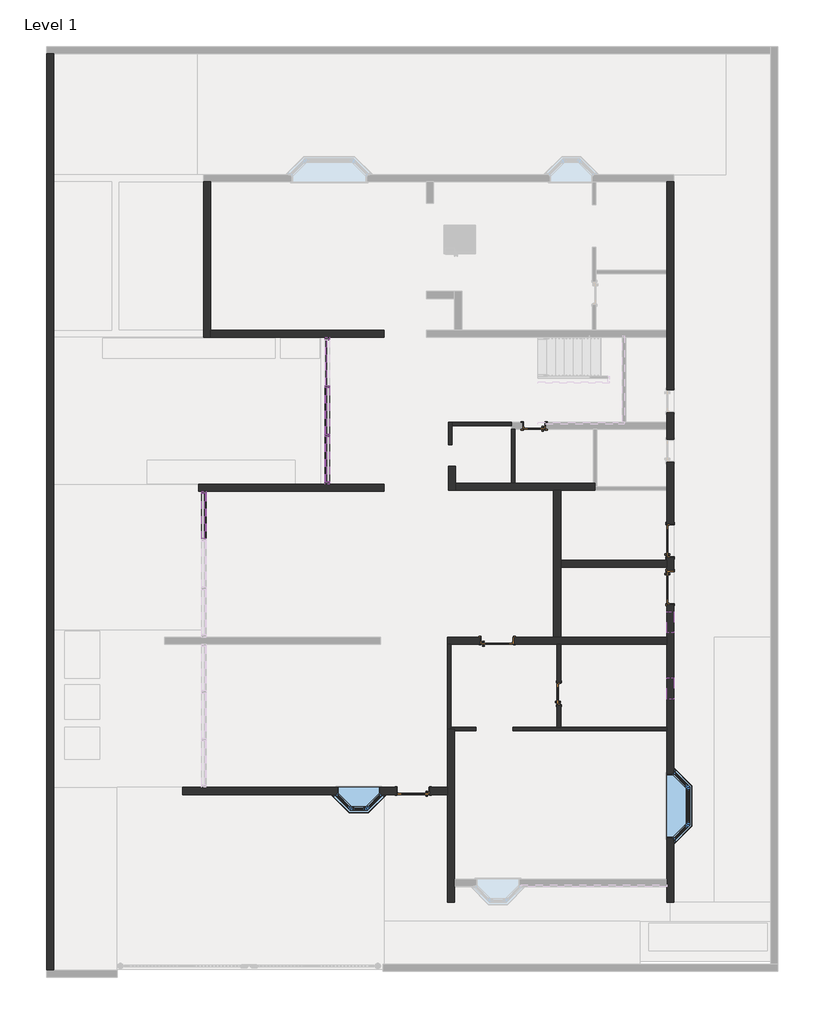
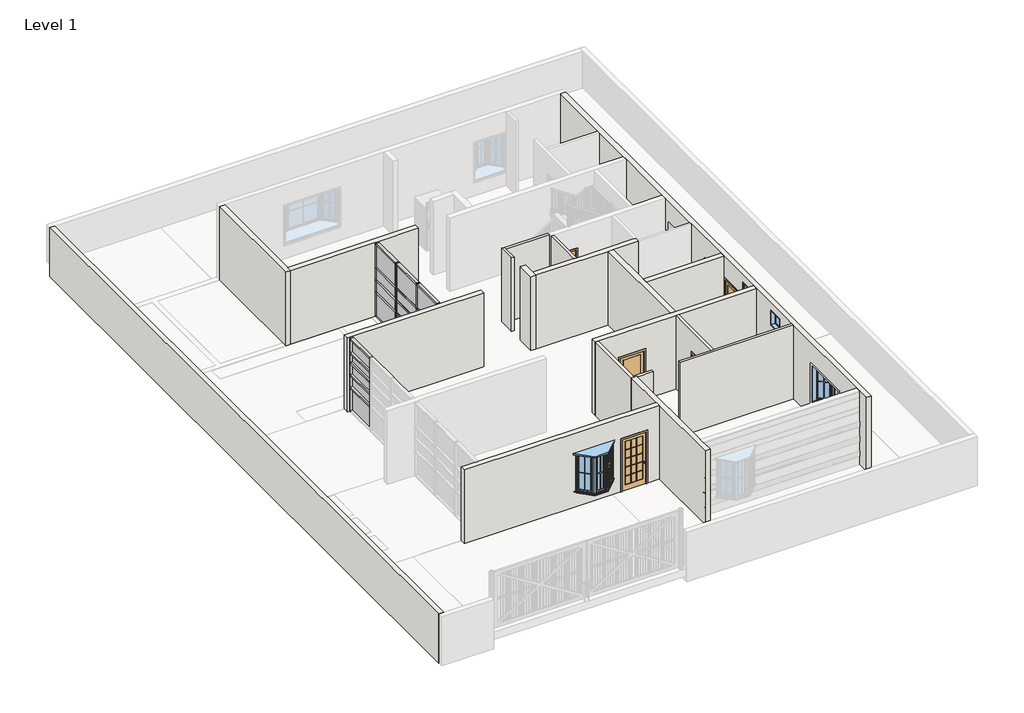
# One storey, part 3 of 5: 38 members, 19 walls, 17 plates, 6 doors, 4 windows.
"""IFC4 building model written with IfcOpenShell, lengths in millimetres."""

from ifc_helpers import new_model, si_unit, frame, origin, origin_with_axes, place, context, project, spatial, polyline, outline, extrude, faceted_brep, transform, mapped, element, save
from components import door_interior_single_1_panel_wood_5fe0af8f, door_interior_single_1_panel_wood_33af59b7, door_89b565b6, door_interior_single_1_panel_wood_secondary_door_3_x_7_9c4ddfbd, door_interior_single_1_panel_wood_secondary_door_3_x_7_1a936fe1, door_interior_single_full_glass_wood_main_glass_door_aaee7461, member_c0a82454, member_10605c90, member_f92b8aa2, member_90750a43, member_f9f7e124, member_161f4059, member_8e09d03a, member_7fd687a9, member_13061b82, member_37fe5cbd, member_7cfea1b5, member_47bfaf8a, system_panel_glazed_751bbe7c, system_panel_glazed_6c2f0e29, system_panel_glazed_201df7ca, system_panel_glazed_b8f86fea, system_panel_glazed_b72ced83, system_panel_glazed_b8338f5c, system_panel_glazed_2a12a50e, system_panel_glazed_2e6a26f2, window_6846e476, window_bay_casement_45_degree_angle_window_4_787d36ed, window_bay_casement_45_degree_angle_window_6_x4_737bffb6

model = new_model("IFC4")

# Units and contexts
model_context = context("Model", 3, world=origin())
ifc_project = project(units=[si_unit("LENGTHUNIT", "METRE", prefix="MILLI")], contexts=[model_context])

# Site, building, storey
site = spatial("IfcSite", under=ifc_project)
building = spatial("IfcBuilding", under=site)
storey = spatial("IfcBuildingStorey", under=building, Name="Level 1", Elevation=0.0)

# Doors
placement = place(None, origin())
door_interior_single_1_panel_wood_shape = door_interior_single_1_panel_wood_5fe0af8f(model_context)
element("IfcDoor", 1, ObjectType="Door-Interior-Single-1_Panel-Wood", at=placement, inside=storey, context=model_context, shape_type="MappedRepresentation", body=[
    mapped(door_interior_single_1_panel_wood_shape, transform((-41259.7380314, 3229.1336027, 0.0), x_axis=(-1.0, 0.0, 0.0), y_axis=(0.0, -1.0, 0.0), z_axis=(0.0, 0.0, 1.0))),
])
door_interior_single_1_panel_wood_2_shape = door_interior_single_1_panel_wood_33af59b7(model_context)
element("IfcDoor", 2, ObjectType="Door-Interior-Single-1_Panel-Wood", at=placement, inside=storey, context=model_context, shape_type="MappedRepresentation", body=[
    mapped(door_interior_single_1_panel_wood_2_shape, transform((-40551.7130314, -4463.8913973, 0.0), x_axis=(0.0, 1.0, 0.0), y_axis=(-1.0, 0.0, 0.0), z_axis=(0.0, 0.0, 1.0))),
])
door_shape = door_89b565b6(model_context)
element("IfcDoor", 3, ObjectType="Door-Interior-Single-1_Panel-Wood : 36\" x 80\"", at=placement, inside=storey, context=model_context, shape_type="MappedRepresentation", body=[
    mapped(door_shape, transform((-42326.5380314, -2943.0663973, 0.0), x_axis=(1.0, 0.0, 0.0), y_axis=(0.0, 1.0, 0.0), z_axis=(0.0, 0.0, 1.0))),
])
door_interior_single_1_panel_wood_secondary_door_3_x_7_shape = door_interior_single_1_panel_wood_secondary_door_3_x_7_9c4ddfbd(model_context)
element("IfcDoor", 4, ObjectType="Door-Interior-Single-1_Panel-Wood : SECONDARY DOOR 3' X 7'", at=placement, inside=storey, context=model_context, shape_type="MappedRepresentation", body=[
    mapped(door_interior_single_1_panel_wood_secondary_door_3_x_7_shape, transform((-37351.3130314, -69.6913973, 0.0), x_axis=(0.0, 1.0, 0.0), y_axis=(-1.0, 0.0, 0.0), z_axis=(0.0, 0.0, 1.0))),
])
door_interior_single_1_panel_wood_secondary_door_3_x_7_2_shape = door_interior_single_1_panel_wood_secondary_door_3_x_7_1a936fe1(model_context)
element("IfcDoor", 5, ObjectType="Door-Interior-Single-1_Panel-Wood : SECONDARY DOOR 3' X 7'", at=placement, inside=storey, context=model_context, shape_type="MappedRepresentation", body=[
    mapped(door_interior_single_1_panel_wood_secondary_door_3_x_7_2_shape, transform((-37351.3130314, -1415.8913973, 0.0), x_axis=(0.0, -1.0, 0.0), y_axis=(1.0, 0.0, 0.0), z_axis=(0.0, 0.0, 1.0))),
])
door_interior_single_full_glass_wood_main_glass_door_shape = door_interior_single_full_glass_wood_main_glass_door_aaee7461(model_context)
element("IfcDoor", 6, ObjectType="Door-Interior-Single-Full Glass-Wood : MAIN GLASS DOOR", at=placement, inside=storey, context=model_context, shape_type="MappedRepresentation", body=[
    mapped(door_interior_single_full_glass_wood_main_glass_door_shape, transform((-44739.5380314, -7261.0663973, 0.0), x_axis=(-1.0, 0.0, 0.0), y_axis=(0.0, -1.0, 0.0), z_axis=(0.0, 0.0, 1.0))),
])

# Members
member_shape = member_c0a82454(model_context)
element("IfcMember", 7, ObjectType="Rectangular Mullion : 2.5\" x 5\" rectangular", at=placement, inside=storey, context=model_context, shape_type="MappedRepresentation", body=[
    mapped(member_shape, transform((-47203.3380314, 5708.8086027, 3048.0), x_axis=(0.0, 0.0, 1.0), y_axis=(1.0, 0.0, 0.0), z_axis=(0.0, 1.0, 0.0))),
])
element("IfcMember", 8, ObjectType="Rectangular Mullion : 2.5\" x 5\" rectangular", at=placement, inside=storey, context=model_context, shape_type="MappedRepresentation", body=[
    mapped(member_shape, transform((-47203.3380314, 2929.6252695, 3048.0), x_axis=(0.0, 0.0, 1.0), y_axis=(1.0, 0.0, 0.0), z_axis=(0.0, 1.0, 0.0))),
])
element("IfcMember", 9, ObjectType="Rectangular Mullion : 2.5\" x 5\" rectangular", at=placement, inside=storey, context=model_context, shape_type="MappedRepresentation", body=[
    mapped(member_shape, transform((-47203.3380314, 1619.4086027, 0.0), x_axis=(0.0, 0.0, -1.0), y_axis=(1.0, 0.0, 0.0), z_axis=(0.0, -1.0, 0.0))),
])
element("IfcMember", 10, ObjectType="Rectangular Mullion : 2.5\" x 5\" rectangular", at=placement, inside=storey, context=model_context, shape_type="MappedRepresentation", body=[
    mapped(member_shape, transform((-47203.3380314, 4398.591936, 0.0), x_axis=(0.0, 0.0, -1.0), y_axis=(1.0, 0.0, 0.0), z_axis=(0.0, -1.0, 0.0))),
])
member_2_shape = member_10605c90(model_context)
element("IfcMember", 11, ObjectType="Rectangular Mullion : 2.5\" x 5\" rectangular", at=placement, inside=storey, context=model_context, shape_type="MappedRepresentation", body=[
    mapped(member_2_shape, transform((-47203.3380314, 4335.091936, 3048.0), x_axis=(0.0, 0.0, 1.0), y_axis=(1.0, 0.0, 0.0), z_axis=(0.0, 1.0, 0.0))),
])
element("IfcMember", 12, ObjectType="Rectangular Mullion : 2.5\" x 5\" rectangular", at=placement, inside=storey, context=model_context, shape_type="MappedRepresentation", body=[
    mapped(member_2_shape, transform((-47203.3380314, 2993.1252695, 0.0), x_axis=(0.0, 0.0, -1.0), y_axis=(1.0, 0.0, 0.0), z_axis=(0.0, -1.0, 0.0))),
])
member_3_shape = member_f92b8aa2(model_context)
element("IfcMember", 13, ObjectType="Rectangular Mullion : 2.5\" x 5\" rectangular", at=placement, inside=storey, context=model_context, shape_type="MappedRepresentation", body=[
    mapped(member_3_shape, transform((-47203.3380314, 4366.841936, 2032.0), x_axis=(0.0, 1.0, 0.0), y_axis=(1.0, 0.0, 0.0), z_axis=(0.0, 0.0, -1.0))),
])
element("IfcMember", 14, ObjectType="Rectangular Mullion : 2.5\" x 5\" rectangular", at=placement, inside=storey, context=model_context, shape_type="MappedRepresentation", body=[
    mapped(member_3_shape, transform((-47203.3380314, 2961.3752695, 2032.0), x_axis=(0.0, 1.0, 0.0), y_axis=(1.0, 0.0, 0.0), z_axis=(0.0, 0.0, -1.0))),
])
member_4_shape = member_90750a43(model_context)
element("IfcMember", 15, ObjectType="Rectangular Mullion : 2.5\" x 5\" rectangular", at=placement, inside=storey, context=model_context, shape_type="MappedRepresentation", body=[
    mapped(member_4_shape, transform((-47203.3380314, 4366.841936, 1016.0), x_axis=(0.0, 1.0, 0.0), y_axis=(1.0, 0.0, 0.0), z_axis=(0.0, 0.0, -1.0))),
])
element("IfcMember", 16, ObjectType="Rectangular Mullion : 2.5\" x 5\" rectangular", at=placement, inside=storey, context=model_context, shape_type="MappedRepresentation", body=[
    mapped(member_4_shape, transform((-47203.3380314, 4366.841936, 1524.0), x_axis=(0.0, 1.0, 0.0), y_axis=(1.0, 0.0, 0.0), z_axis=(0.0, 0.0, -1.0))),
])
element("IfcMember", 17, ObjectType="Rectangular Mullion : 2.5\" x 5\" rectangular", at=placement, inside=storey, context=model_context, shape_type="MappedRepresentation", body=[
    mapped(member_4_shape, transform((-47203.3380314, 2961.3752695, 1016.0), x_axis=(0.0, 1.0, 0.0), y_axis=(1.0, 0.0, 0.0), z_axis=(0.0, 0.0, -1.0))),
])
element("IfcMember", 18, ObjectType="Rectangular Mullion : 2.5\" x 5\" rectangular", at=placement, inside=storey, context=model_context, shape_type="MappedRepresentation", body=[
    mapped(member_4_shape, transform((-47203.3380314, 2961.3752695, 1524.0), x_axis=(0.0, 1.0, 0.0), y_axis=(1.0, 0.0, 0.0), z_axis=(0.0, 0.0, -1.0))),
])
element("IfcMember", 19, ObjectType="Rectangular Mullion : 2.5\" x 5\" rectangular", at=placement, inside=storey, context=model_context, shape_type="MappedRepresentation", body=[
    mapped(member_3_shape, transform((-47203.3380314, 4366.841936, 0.0), x_axis=(0.0, 1.0, 0.0), y_axis=(1.0, 0.0, 0.0), z_axis=(0.0, 0.0, -1.0))),
])
element("IfcMember", 20, ObjectType="Rectangular Mullion : 2.5\" x 5\" rectangular", at=placement, inside=storey, context=model_context, shape_type="MappedRepresentation", body=[
    mapped(member_3_shape, transform((-47203.3380314, 2961.3752695, 0.0), x_axis=(0.0, 1.0, 0.0), y_axis=(1.0, 0.0, 0.0), z_axis=(0.0, 0.0, -1.0))),
])
member_5_shape = member_f9f7e124(model_context)
element("IfcMember", 21, ObjectType="Rectangular Mullion : 2.5\" x 5\" rectangular", at=placement, inside=storey, context=model_context, shape_type="MappedRepresentation", body=[
    mapped(member_5_shape, transform((-47203.3380314, 2929.6252695, 1016.0), x_axis=(0.0, 0.0, 1.0), y_axis=(1.0, 0.0, 0.0), z_axis=(0.0, 1.0, 0.0))),
])
element("IfcMember", 22, ObjectType="Rectangular Mullion : 2.5\" x 5\" rectangular", at=placement, inside=storey, context=model_context, shape_type="MappedRepresentation", body=[
    mapped(member_5_shape, transform((-47203.3380314, 2929.6252695, 2032.0), x_axis=(0.0, 0.0, 1.0), y_axis=(1.0, 0.0, 0.0), z_axis=(0.0, 1.0, 0.0))),
])
element("IfcMember", 23, ObjectType="Rectangular Mullion : 2.5\" x 5\" rectangular", at=placement, inside=storey, context=model_context, shape_type="MappedRepresentation", body=[
    mapped(member_5_shape, transform((-47203.3380314, 2929.6252695, 1524.0), x_axis=(0.0, 0.0, 1.0), y_axis=(1.0, 0.0, 0.0), z_axis=(0.0, 1.0, 0.0))),
])
member_6_shape = member_161f4059(model_context)
element("IfcMember", 24, ObjectType="Rectangular Mullion : 2.5\" x 5\" rectangular", at=placement, inside=storey, context=model_context, shape_type="MappedRepresentation", body=[
    mapped(member_6_shape, transform((-47203.3380314, 4335.091936, 1016.0), x_axis=(0.0, 0.0, 1.0), y_axis=(1.0, 0.0, 0.0), z_axis=(0.0, 1.0, 0.0))),
])
element("IfcMember", 25, ObjectType="Rectangular Mullion : 2.5\" x 5\" rectangular", at=placement, inside=storey, context=model_context, shape_type="MappedRepresentation", body=[
    mapped(member_6_shape, transform((-47203.3380314, 4335.091936, 2032.0), x_axis=(0.0, 0.0, 1.0), y_axis=(1.0, 0.0, 0.0), z_axis=(0.0, 1.0, 0.0))),
])
element("IfcMember", 26, ObjectType="Rectangular Mullion : 2.5\" x 5\" rectangular", at=placement, inside=storey, context=model_context, shape_type="MappedRepresentation", body=[
    mapped(member_6_shape, transform((-47203.3380314, 4335.091936, 1524.0), x_axis=(0.0, 0.0, 1.0), y_axis=(1.0, 0.0, 0.0), z_axis=(0.0, 1.0, 0.0))),
])
member_7_shape = member_8e09d03a(model_context)
element("IfcMember", 27, ObjectType="Rectangular Mullion : 2.5\" x 5\" rectangular", at=placement, inside=storey, context=model_context, shape_type="MappedRepresentation", body=[
    mapped(member_7_shape, transform((-47203.3380314, 5772.3086027, 0.0), x_axis=(0.0, 1.0, 0.0), y_axis=(1.0, 0.0, 0.0), z_axis=(0.0, 0.0, -1.0))),
])
element("IfcMember", 28, ObjectType="Rectangular Mullion : 2.5\" x 5\" rectangular", at=placement, inside=storey, context=model_context, shape_type="MappedRepresentation", body=[
    mapped(member_7_shape, transform((-47203.3380314, 1555.9086027, 3048.0), x_axis=(0.0, -1.0, 0.0), y_axis=(1.0, 0.0, 0.0), z_axis=(0.0, 0.0, 1.0))),
])
member_8_shape = member_7fd687a9(model_context)
element("IfcMember", 29, ObjectType="Rectangular Mullion : 2.5\" x 5\" rectangular", at=placement, inside=storey, context=model_context, shape_type="MappedRepresentation", body=[
    mapped(member_8_shape, transform((-47203.3380314, 5772.3086027, 1016.0), x_axis=(0.0, 1.0, 0.0), y_axis=(1.0, 0.0, 0.0), z_axis=(0.0, 0.0, -1.0))),
])
element("IfcMember", 30, ObjectType="Rectangular Mullion : 2.5\" x 5\" rectangular", at=placement, inside=storey, context=model_context, shape_type="MappedRepresentation", body=[
    mapped(member_8_shape, transform((-47203.3380314, 5772.3086027, 1524.0), x_axis=(0.0, 1.0, 0.0), y_axis=(1.0, 0.0, 0.0), z_axis=(0.0, 0.0, -1.0))),
])
element("IfcMember", 31, ObjectType="Rectangular Mullion : 2.5\" x 5\" rectangular", at=placement, inside=storey, context=model_context, shape_type="MappedRepresentation", body=[
    mapped(member_7_shape, transform((-47203.3380314, 1555.9086027, 1016.0), x_axis=(0.0, -1.0, 0.0), y_axis=(1.0, 0.0, 0.0), z_axis=(0.0, 0.0, 1.0))),
])
element("IfcMember", 32, ObjectType="Rectangular Mullion : 2.5\" x 5\" rectangular", at=placement, inside=storey, context=model_context, shape_type="MappedRepresentation", body=[
    mapped(member_8_shape, transform((-47203.3380314, 1555.9086027, 2032.0), x_axis=(0.0, -1.0, 0.0), y_axis=(1.0, 0.0, 0.0), z_axis=(0.0, 0.0, 1.0))),
])
element("IfcMember", 33, ObjectType="Rectangular Mullion : 2.5\" x 5\" rectangular", at=placement, inside=storey, context=model_context, shape_type="MappedRepresentation", body=[
    mapped(member_8_shape, transform((-47203.3380314, 1555.9086027, 1524.0), x_axis=(0.0, -1.0, 0.0), y_axis=(1.0, 0.0, 0.0), z_axis=(0.0, 0.0, 1.0))),
])
element("IfcMember", 34, ObjectType="Rectangular Mullion : 2.5\" x 5\" rectangular", at=placement, inside=storey, context=model_context, shape_type="MappedRepresentation", body=[
    mapped(member_7_shape, transform((-47203.3380314, 5772.3086027, 2032.0), x_axis=(0.0, 1.0, 0.0), y_axis=(1.0, 0.0, 0.0), z_axis=(0.0, 0.0, -1.0))),
])
member_9_shape = member_13061b82(model_context)
element("IfcMember", 35, ObjectType="Rectangular Mullion : 2.5\" x 5\" rectangular", at=placement, inside=storey, context=model_context, shape_type="MappedRepresentation", body=[
    mapped(member_9_shape, transform((-50759.3380314, 1289.2086027, 3048.0), x_axis=(0.0, 0.0, 1.0), y_axis=(1.0, 0.0, 0.0), z_axis=(0.0, 1.0, 0.0))),
])
member_10_shape = member_37fe5cbd(model_context)
element("IfcMember", 36, ObjectType="Rectangular Mullion : 2.5\" x 5\" rectangular", at=placement, inside=storey, context=model_context, shape_type="MappedRepresentation", body=[
    mapped(member_10_shape, transform((-50759.3380314, 1289.2086027, 1016.0), x_axis=(0.0, 0.0, 1.0), y_axis=(1.0, 0.0, 0.0), z_axis=(0.0, 1.0, 0.0))),
])
element("IfcMember", 37, ObjectType="Rectangular Mullion : 2.5\" x 5\" rectangular", at=placement, inside=storey, context=model_context, shape_type="MappedRepresentation", body=[
    mapped(member_10_shape, transform((-50759.3380314, 1289.2086027, 2032.0), x_axis=(0.0, 0.0, 1.0), y_axis=(1.0, 0.0, 0.0), z_axis=(0.0, 1.0, 0.0))),
])
element("IfcMember", 38, ObjectType="Rectangular Mullion : 2.5\" x 5\" rectangular", at=placement, inside=storey, context=model_context, shape_type="MappedRepresentation", body=[
    mapped(member_10_shape, transform((-50759.3380314, 1289.2086027, 1524.0), x_axis=(0.0, 0.0, 1.0), y_axis=(1.0, 0.0, 0.0), z_axis=(0.0, 1.0, 0.0))),
])
element("IfcMember", 39, ObjectType="Rectangular Mullion : 2.5\" x 5\" rectangular", at=placement, inside=storey, context=model_context, shape_type="MappedRepresentation", body=[
    mapped(member_10_shape, transform((-50759.3380314, 1289.2086027, 2438.4), x_axis=(0.0, 0.0, 1.0), y_axis=(1.0, 0.0, 0.0), z_axis=(0.0, 1.0, 0.0))),
])
element("IfcMember", 40, ObjectType="Rectangular Mullion : 2.5\" x 5\" rectangular", at=placement, inside=storey, context=model_context, shape_type="MappedRepresentation", body=[
    mapped(member_7_shape, transform((-50759.3380314, 1352.7086027, 0.0), x_axis=(0.0, 1.0, 0.0), y_axis=(1.0, 0.0, 0.0), z_axis=(0.0, 0.0, -1.0))),
])
element("IfcMember", 41, ObjectType="Rectangular Mullion : 2.5\" x 5\" rectangular", at=placement, inside=storey, context=model_context, shape_type="MappedRepresentation", body=[
    mapped(member_8_shape, transform((-50759.3380314, 1352.7086027, 1016.0), x_axis=(0.0, 1.0, 0.0), y_axis=(1.0, 0.0, 0.0), z_axis=(0.0, 0.0, -1.0))),
])
element("IfcMember", 42, ObjectType="Rectangular Mullion : 2.5\" x 5\" rectangular", at=placement, inside=storey, context=model_context, shape_type="MappedRepresentation", body=[
    mapped(member_8_shape, transform((-50759.3380314, 1352.7086027, 1524.0), x_axis=(0.0, 1.0, 0.0), y_axis=(1.0, 0.0, 0.0), z_axis=(0.0, 0.0, -1.0))),
])
member_11_shape = member_7cfea1b5(model_context)
element("IfcMember", 43, ObjectType="Rectangular Mullion : 2.5\" x 5\" rectangular", at=placement, inside=storey, context=model_context, shape_type="MappedRepresentation", body=[
    mapped(member_11_shape, transform((-50759.3380314, 1352.7086027, 2032.0), x_axis=(0.0, 1.0, 0.0), y_axis=(1.0, 0.0, 0.0), z_axis=(0.0, 0.0, -1.0))),
])
member_12_shape = member_47bfaf8a(model_context)
element("IfcMember", 44, ObjectType="Rectangular Mullion : 2.5\" x 5\" rectangular", at=placement, inside=storey, context=model_context, shape_type="MappedRepresentation", body=[
    mapped(member_12_shape, transform((-50759.3380314, 1352.7086027, 2438.4), x_axis=(0.0, 1.0, 0.0), y_axis=(1.0, 0.0, 0.0), z_axis=(0.0, 0.0, -1.0))),
])

# Plates
system_panel_glazed_shape = system_panel_glazed_751bbe7c(model_context)
element("IfcPlate", 45, ObjectType="System Panel : Glazed", at=placement, inside=storey, context=model_context, shape_type="MappedRepresentation", body=[
    mapped(system_panel_glazed_shape, transform((-47203.3380314, 2274.5169361, 63.5), x_axis=(0.0, 1.0, 0.0), y_axis=(-1.0, 0.0, 0.0), z_axis=(0.0, 0.0, 1.0))),
])
element("IfcPlate", 46, ObjectType="System Panel : Glazed", at=placement, inside=storey, context=model_context, shape_type="MappedRepresentation", body=[
    mapped(system_panel_glazed_shape, transform((-47203.3380314, 5053.7002694, 63.5), x_axis=(0.0, 1.0, 0.0), y_axis=(-1.0, 0.0, 0.0), z_axis=(0.0, 0.0, 1.0))),
])
element("IfcPlate", 47, ObjectType="System Panel : Glazed", at=placement, inside=storey, context=model_context, shape_type="MappedRepresentation", body=[
    mapped(system_panel_glazed_shape, transform((-47203.3380314, 2274.5169361, 2063.75), x_axis=(0.0, 1.0, 0.0), y_axis=(-1.0, 0.0, 0.0), z_axis=(0.0, 0.0, 1.0))),
])
element("IfcPlate", 48, ObjectType="System Panel : Glazed", at=placement, inside=storey, context=model_context, shape_type="MappedRepresentation", body=[
    mapped(system_panel_glazed_shape, transform((-47203.3380314, 5053.7002694, 2063.75), x_axis=(0.0, 1.0, 0.0), y_axis=(-1.0, 0.0, 0.0), z_axis=(0.0, 0.0, 1.0))),
])
system_panel_glazed_2_shape = system_panel_glazed_6c2f0e29(model_context)
element("IfcPlate", 49, ObjectType="System Panel : Glazed", at=placement, inside=storey, context=model_context, shape_type="MappedRepresentation", body=[
    mapped(system_panel_glazed_2_shape, transform((-47203.3380314, 3664.1086027, 63.5), x_axis=(0.0, 1.0, 0.0), y_axis=(-1.0, 0.0, 0.0), z_axis=(0.0, 0.0, 1.0))),
])
element("IfcPlate", 50, ObjectType="System Panel : Glazed", at=placement, inside=storey, context=model_context, shape_type="MappedRepresentation", body=[
    mapped(system_panel_glazed_2_shape, transform((-47203.3380314, 3664.1086027, 2063.75), x_axis=(0.0, 1.0, 0.0), y_axis=(-1.0, 0.0, 0.0), z_axis=(0.0, 0.0, 1.0))),
])
system_panel_glazed_3_shape = system_panel_glazed_201df7ca(model_context)
element("IfcPlate", 51, ObjectType="System Panel : Glazed", at=placement, inside=storey, context=model_context, shape_type="MappedRepresentation", body=[
    mapped(system_panel_glazed_3_shape, transform((-47203.3380314, 2274.5169361, 1047.75), x_axis=(0.0, 1.0, 0.0), y_axis=(-1.0, 0.0, 0.0), z_axis=(0.0, 0.0, 1.0))),
])
element("IfcPlate", 52, ObjectType="System Panel : Glazed", at=placement, inside=storey, context=model_context, shape_type="MappedRepresentation", body=[
    mapped(system_panel_glazed_3_shape, transform((-47203.3380314, 5053.7002694, 1047.75), x_axis=(0.0, 1.0, 0.0), y_axis=(-1.0, 0.0, 0.0), z_axis=(0.0, 0.0, 1.0))),
])
element("IfcPlate", 53, ObjectType="System Panel : Glazed", at=placement, inside=storey, context=model_context, shape_type="MappedRepresentation", body=[
    mapped(system_panel_glazed_3_shape, transform((-47203.3380314, 2274.5169361, 1555.75), x_axis=(0.0, 1.0, 0.0), y_axis=(-1.0, 0.0, 0.0), z_axis=(0.0, 0.0, 1.0))),
])
element("IfcPlate", 54, ObjectType="System Panel : Glazed", at=placement, inside=storey, context=model_context, shape_type="MappedRepresentation", body=[
    mapped(system_panel_glazed_3_shape, transform((-47203.3380314, 5053.7002694, 1555.75), x_axis=(0.0, 1.0, 0.0), y_axis=(-1.0, 0.0, 0.0), z_axis=(0.0, 0.0, 1.0))),
])
system_panel_glazed_4_shape = system_panel_glazed_b8f86fea(model_context)
element("IfcPlate", 55, ObjectType="System Panel : Glazed", at=placement, inside=storey, context=model_context, shape_type="MappedRepresentation", body=[
    mapped(system_panel_glazed_4_shape, transform((-47203.3380314, 3664.1086027, 1047.75), x_axis=(0.0, 1.0, 0.0), y_axis=(-1.0, 0.0, 0.0), z_axis=(0.0, 0.0, 1.0))),
])
element("IfcPlate", 56, ObjectType="System Panel : Glazed", at=placement, inside=storey, context=model_context, shape_type="MappedRepresentation", body=[
    mapped(system_panel_glazed_4_shape, transform((-47203.3380314, 3664.1086027, 1555.75), x_axis=(0.0, 1.0, 0.0), y_axis=(-1.0, 0.0, 0.0), z_axis=(0.0, 0.0, 1.0))),
])
system_panel_glazed_5_shape = system_panel_glazed_b72ced83(model_context)
element("IfcPlate", 57, ObjectType="System Panel : Glazed", at=placement, inside=storey, context=model_context, shape_type="MappedRepresentation", body=[
    mapped(system_panel_glazed_5_shape, transform((-50759.3380314, 638.3336027, 63.5), x_axis=(0.0, 1.0, 0.0), y_axis=(-1.0, 0.0, 0.0), z_axis=(0.0, 0.0, 1.0))),
])
system_panel_glazed_6_shape = system_panel_glazed_b8338f5c(model_context)
element("IfcPlate", 58, ObjectType="System Panel : Glazed", at=placement, inside=storey, context=model_context, shape_type="MappedRepresentation", body=[
    mapped(system_panel_glazed_6_shape, transform((-50759.3380314, 638.3336027, 1047.75), x_axis=(0.0, 1.0, 0.0), y_axis=(-1.0, 0.0, 0.0), z_axis=(0.0, 0.0, 1.0))),
])
element("IfcPlate", 59, ObjectType="System Panel : Glazed", at=placement, inside=storey, context=model_context, shape_type="MappedRepresentation", body=[
    mapped(system_panel_glazed_6_shape, transform((-50759.3380314, 638.3336027, 1555.75), x_axis=(0.0, 1.0, 0.0), y_axis=(-1.0, 0.0, 0.0), z_axis=(0.0, 0.0, 1.0))),
])
system_panel_glazed_7_shape = system_panel_glazed_2a12a50e(model_context)
element("IfcPlate", 60, ObjectType="System Panel : Glazed", at=placement, inside=storey, context=model_context, shape_type="MappedRepresentation", body=[
    mapped(system_panel_glazed_7_shape, transform((-50759.3380314, 638.3336027, 2063.75), x_axis=(0.0, 1.0, 0.0), y_axis=(-1.0, 0.0, 0.0), z_axis=(0.0, 0.0, 1.0))),
])
system_panel_glazed_8_shape = system_panel_glazed_2e6a26f2(model_context)
element("IfcPlate", 61, ObjectType="System Panel : Glazed", at=placement, inside=storey, context=model_context, shape_type="MappedRepresentation", body=[
    mapped(system_panel_glazed_8_shape, transform((-50759.3380314, 638.3336027, 2470.15), x_axis=(0.0, 1.0, 0.0), y_axis=(-1.0, 0.0, 0.0), z_axis=(0.0, 0.0, 1.0))),
])

# Walls
element("IfcWall", 62, ObjectType="INNER WALL 4\"", at=placement, inside=storey, context=model_context, shape_type="SweptSolid", body=[
    extrude(outline(polyline([(-41920.1380314, 1581.3086027), (-41920.1380314, 3130.7086027), (-41818.5380314, 3130.7086027), (-41818.5380314, 1581.3086027), (-41920.1380314, 1581.3086027)])), origin_with_axes(), (0.0, 0.0, 1.0), 3048.0),
])
element("IfcWall", 63, ObjectType="INNER WALL 4\"", at=placement, inside=storey, context=model_context, shape_type="Brep", body=[
    faceted_brep([(-43748.9380314, -3041.4913973, 0.0), (-43748.9380314, -5479.8913973, 0.0), (-43748.9380314, -5479.8913973, 3048.0), (-43748.9380314, -3041.4913973, 3048.0), (-43647.3380314, -3041.4913973, 0.0), (-43647.3380314, -3041.4913973, 3048.0), (-43647.3380314, -5429.0913973, 3048.0), (-43647.3380314, -5479.8913973, 3048.0), (-43647.3380314, -5479.8913973, 0.0), (-43647.3380314, -5429.0913973, 0.0)], [[[0, 1, 2, 3]], [[4, 5, 6, 7, 8, 9]], [[1, 0, 4, 9, 8]], [[2, 1, 8, 7]], [[3, 2, 7, 6, 5]], [[0, 3, 5, 4]]]),
])
element("IfcWall", 64, ObjectType="INNER WALL 4\"", at=placement, inside=storey, context=model_context, shape_type="SweptSolid", body=[
    extrude(outline(polyline([(-43647.3380314, -5429.0913973), (-42936.1380314, -5429.0913973), (-42936.1380314, -5530.6913973), (-43545.7380314, -5530.6913973), (-43545.7380314, -5479.8913973), (-43647.3380314, -5479.8913973), (-43647.3380314, -5429.0913973)])), origin_with_axes(), (0.0, 0.0, 1.0), 3048.0),
])
element("IfcWall", 65, ObjectType="INNER WALL 4\"", at=placement, inside=storey, context=model_context, shape_type="Brep", body=[
    faceted_brep([(-41869.3380314, -5530.6913973, 0.0), (-37449.7380314, -5530.6913973, 0.0), (-37449.7380314, -5530.6913973, 3048.0), (-41869.3380314, -5530.6913973, 3048.0), (-41869.3380314, -5429.0913973, 0.0), (-41869.3380314, -5429.0913973, 3048.0), (-40599.3380314, -5429.0913973, 3048.0), (-40497.7380314, -5429.0913973, 3048.0), (-37449.7380314, -5429.0913973, 3048.0), (-37449.7380314, -5429.0913973, 0.0), (-40497.7380314, -5429.0913973, 0.0), (-40599.3380314, -5429.0913973, 0.0)], [[[0, 1, 2, 3]], [[4, 5, 6, 7, 8, 9, 10, 11]], [[1, 0, 4, 11, 10, 9]], [[3, 2, 8, 7, 6, 5]], [[0, 3, 5, 4]], [[2, 1, 9, 8]]]),
])
element("IfcWall", 66, ObjectType="INNER WALL 4\"", at=placement, inside=storey, context=model_context, shape_type="SweptSolid", body=[
    extrude(outline(polyline([(-5429.0913973, 3048.0), (-3041.4913973, 3048.0), (-3041.4913973, 0.0), (-4133.6913973, 0.0), (-4133.6913973, 2159.0), (-4794.0913973, 2159.0), (-4794.0913973, 0.0), (-5429.0913973, 0.0), (-5429.0913973, 3048.0)])), frame((-40599.3380314, 0.0, 0.0), z_axis=(1.0, 0.0, 0.0), x_axis=(0.0, 1.0, 0.0)), (0.0, 0.0, 1.0), 101.6),
])
element("IfcWall", 67, ObjectType="INNER WALL 4\"", at=placement, inside=storey, context=model_context, shape_type="Brep", body=[
    faceted_brep([(-43621.9380314, 2686.2086027, 0.0), (-43621.9380314, 3232.3086027, 0.0), (-43621.9380314, 3333.9086027, 0.0), (-43621.9380314, 3333.9086027, 3048.0), (-43621.9380314, 3232.3086027, 3048.0), (-43621.9380314, 2686.2086027, 3048.0), (-43723.5380314, 2686.2086027, 0.0), (-43723.5380314, 2686.2086027, 3048.0), (-43723.5380314, 3333.9086027, 3048.0), (-43723.5380314, 3333.9086027, 0.0)], [[[0, 1, 2, 3, 4, 5]], [[6, 7, 8, 9]], [[2, 1, 0, 6, 9]], [[5, 4, 3, 8, 7]], [[0, 5, 7, 6]], [[3, 2, 9, 8]]]),
])
element("IfcWall", 68, ObjectType="INNER WALL 4\"", at=placement, inside=storey, context=model_context, shape_type="SweptSolid", body=[
    extrude(outline(polyline([(-41920.1380314, 3232.3086027), (-43621.9380314, 3232.3086027), (-43621.9380314, 3333.9086027), (-41920.1380314, 3333.9086027), (-41920.1380314, 3232.3086027)])), origin_with_axes(), (0.0, 0.0, 1.0), 3048.0),
])
element("IfcWall", 69, ObjectType="OUTER WALL 8\"", at=placement, inside=storey, context=model_context, shape_type="Brep", body=[
    faceted_brep([(-50759.3380314, 10242.7086027, 0.0), (-50759.3380314, 5772.3086027, 0.0), (-50759.3380314, 5772.3086027, 3048.0), (-50759.3380314, 10242.7086027, 3048.0), (-50556.1380314, 10242.7086027, 0.0), (-50556.1380314, 10242.7086027, 3048.0), (-50556.1380314, 5975.5086027, 3048.0), (-50556.1380314, 5772.3086027, 3048.0), (-50556.1380314, 5772.3086027, 0.0), (-50556.1380314, 5975.5086027, 0.0)], [[[0, 1, 2, 3]], [[4, 5, 6, 7, 8, 9]], [[1, 0, 4, 9, 8]], [[3, 2, 7, 6, 5]], [[0, 3, 5, 4]], [[2, 1, 8, 7]]]),
])
element("IfcWall", 70, ObjectType="OUTER WALL 8\"", at=placement, inside=storey, context=model_context, shape_type="Brep", body=[
    faceted_brep([(-45577.7380314, 5975.5086027, 0.0), (-50556.1380314, 5975.5086027, 0.0), (-50556.1380314, 5975.5086027, 3048.0), (-45577.7380314, 5975.5086027, 3048.0), (-45577.7380314, 5772.3086027, 0.0), (-45577.7380314, 5772.3086027, 3048.0), (-47203.3380314, 5772.3086027, 3048.0), (-47406.5380314, 5772.3086027, 3048.0), (-50556.1380314, 5772.3086027, 3048.0), (-50556.1380314, 5772.3086027, 0.0), (-47406.5380314, 5772.3086027, 0.0), (-47203.3380314, 5772.3086027, 0.0)], [[[0, 1, 2, 3]], [[4, 5, 6, 7, 8, 9, 10, 11]], [[1, 0, 4, 11, 10, 9]], [[3, 2, 8, 7, 6, 5]], [[0, 3, 5, 4]], [[2, 1, 9, 8]]]),
])
element("IfcWall", 71, ObjectType="OUTER WALL 8\"", at=placement, inside=storey, context=model_context, shape_type="SweptSolid", body=[
    extrude(outline(polyline([(-50905.3880314, 1555.9086027), (-45577.7380314, 1555.9086027), (-45577.7380314, 1352.7086027), (-50905.3880314, 1352.7086027), (-50905.3880314, 1555.9086027)])), origin_with_axes(), (0.0, 0.0, 1.0), 3048.0),
])
element("IfcWall", 72, ObjectType="OUTER WALL 8\"", at=placement, inside=storey, context=model_context, shape_type="Brep", body=[
    faceted_brep([(-43748.9380314, -7359.4913973, 3048.0), (-51368.9380314, -7359.4913973, 3048.0), (-51368.9380314, -7359.4913973, 0.0), (-45222.1380314, -7359.4913973, 0.0), (-45222.1380314, -7359.4913973, 2159.0), (-44256.9380314, -7359.4913973, 2159.0), (-44256.9380314, -7359.4913973, 0.0), (-43748.9380314, -7359.4913973, 0.0), (-46960.6294401, -7359.4913973, 2184.4), (-45642.6466227, -7359.4913973, 2184.4), (-45642.6466227, -7359.4913973, 609.6), (-46960.6294401, -7359.4913973, 609.6), (-51368.9380314, -7156.2913973, 3048.0), (-43748.9380314, -7156.2913973, 3048.0), (-43748.9380314, -7156.2913973, 0.0), (-44256.9380314, -7156.2913973, 0.0), (-44256.9380314, -7156.2913973, 2159.0), (-45222.1380314, -7156.2913973, 2159.0), (-45222.1380314, -7156.2913973, 0.0), (-51368.9380314, -7156.2913973, 0.0), (-45692.0380314, -7156.2913973, 2184.4), (-46911.2380314, -7156.2913973, 2184.4), (-46911.2380314, -7156.2913973, 609.6), (-45692.0380314, -7156.2913973, 609.6), (-45692.0380314, -7310.0999886, 2184.4), (-46911.2380314, -7310.0999886, 2184.4), (-45692.0380314, -7310.0999886, 609.6), (-46911.2380314, -7310.0999886, 609.6)], [[[0, 1, 2, 3, 4, 5, 6, 7], [8, 9, 10, 11]], [[12, 13, 14, 15, 16, 17, 18, 19], [20, 21, 22, 23]], [[2, 19, 18, 3]], [[14, 7, 6, 15]], [[1, 0, 13, 12]], [[2, 1, 12, 19]], [[0, 7, 14, 13]], [[17, 4, 3, 18]], [[4, 17, 16, 5]], [[5, 16, 15, 6]], [[24, 9, 8, 25, 21, 20]], [[26, 23, 22, 27, 11, 10]], [[24, 20, 23, 26]], [[21, 25, 27, 22]], [[25, 8, 11, 27]], [[9, 24, 26, 10]]]),
])
element("IfcWall", 73, ObjectType="OUTER WALL 8\"", at=placement, inside=storey, context=model_context, shape_type="Brep", body=[
    faceted_brep([(-43545.7380314, -10458.2913973, 0.0), (-43545.7380314, -10001.0913973, 0.0), (-43545.7380314, -9797.8913973, 0.0), (-43545.7380314, -5530.6913973, 0.0), (-43545.7380314, -5479.8913973, 0.0), (-43545.7380314, -5479.8913973, 3048.0), (-43545.7380314, -5530.6913973, 3048.0), (-43545.7380314, -9797.8913973, 3048.0), (-43545.7380314, -10001.0913973, 3048.0), (-43545.7380314, -10458.2913973, 3048.0), (-43748.9380314, -10458.2913973, 0.0), (-43748.9380314, -10458.2913973, 3048.0), (-43748.9380314, -7359.4913973, 3048.0), (-43748.9380314, -7156.2913973, 3048.0), (-43748.9380314, -5479.8913973, 3048.0), (-43748.9380314, -5479.8913973, 0.0), (-43748.9380314, -7156.2913973, 0.0), (-43748.9380314, -7359.4913973, 0.0), (-43647.3380314, -5479.8913973, 0.0), (-43647.3380314, -5479.8913973, 3048.0)], [[[0, 1, 2, 3, 4, 5, 6, 7, 8, 9]], [[10, 11, 12, 13, 14, 15, 16, 17]], [[4, 3, 2, 1, 0, 10, 17, 16, 15, 18]], [[5, 4, 18, 15, 14, 19]], [[9, 8, 7, 6, 5, 19, 14, 13, 12, 11]], [[0, 9, 11, 10]]]),
])
element("IfcWall", 74, ObjectType="OUTER WALL 8\"", at=placement, inside=storey, context=model_context, shape_type="Brep", body=[
    faceted_brep([(-37246.5380314, 10242.7086027, 3048.0), (-37246.5380314, -10458.2913973, 3048.0), (-37246.5380314, -10458.2913973, 0.0), (-37246.5380314, -1898.4913973, 0.0), (-37246.5380314, -1898.4913973, 2159.0), (-37246.5380314, -933.2913973, 2159.0), (-37246.5380314, -933.2913973, 0.0), (-37246.5380314, -552.2913973, 0.0), (-37246.5380314, -552.2913973, 2159.0), (-37246.5380314, 412.9086027, 2159.0), (-37246.5380314, 412.9086027, 0.0), (-37246.5380314, 2190.9086027, 0.0), (-37246.5380314, 2190.9086027, 2159.0), (-37246.5380314, 2851.3086027, 2159.0), (-37246.5380314, 2851.3086027, 0.0), (-37246.5380314, 3613.3086027, 0.0), (-37246.5380314, 3613.3086027, 2159.0), (-37246.5380314, 4273.7086027, 2159.0), (-37246.5380314, 4273.7086027, 0.0), (-37246.5380314, 10242.7086027, 0.0), (-37246.5380314, -8653.4828059, 2184.4), (-37246.5380314, -6725.8999886, 2184.4), (-37246.5380314, -6725.8999886, 609.6), (-37246.5380314, -8653.4828059, 609.6), (-37246.5380314, -4616.2913973, 2133.6), (-37246.5380314, -4616.2913973, 2743.2), (-37246.5380314, -4006.6913973, 2743.2), (-37246.5380314, -4006.6913973, 2133.6), (-37246.5380314, -2101.6913973, 2743.2), (-37246.5380314, -2101.6913973, 2133.6), (-37246.5380314, -2711.2913973, 2133.6), (-37246.5380314, -2711.2913973, 2743.2), (-37449.7380314, -10458.2913973, 3048.0), (-37449.7380314, -10001.0913973, 3048.0), (-37449.7380314, -9797.8913973, 3048.0), (-37449.7380314, -5530.6913973, 3048.0), (-37449.7380314, -5429.0913973, 3048.0), (-37449.7380314, -3041.4913973, 3048.0), (-37449.7380314, -2838.2913973, 3048.0), (-37449.7380314, -831.6913973, 3048.0), (-37449.7380314, -628.4913973, 3048.0), (-37449.7380314, 1378.1086027, 3048.0), (-37449.7380314, 1479.7086027, 3048.0), (-37449.7380314, 3130.7086027, 3048.0), (-37449.7380314, 3333.9086027, 3048.0), (-37449.7380314, 5772.3086027, 3048.0), (-37449.7380314, 5975.5086027, 3048.0), (-37449.7380314, 7601.1086027, 3048.0), (-37449.7380314, 7702.7086027, 3048.0), (-37449.7380314, 10242.7086027, 3048.0), (-37449.7380314, 10242.7086027, 0.0), (-37449.7380314, 7702.7086027, 0.0), (-37449.7380314, 7601.1086027, 0.0), (-37449.7380314, 5975.5086027, 0.0), (-37449.7380314, 5772.3086027, 0.0), (-37449.7380314, 4273.7086027, 0.0), (-37449.7380314, 4273.7086027, 2159.0), (-37449.7380314, 3613.3086027, 2159.0), (-37449.7380314, 3613.3086027, 0.0), (-37449.7380314, 3333.9086027, 0.0), (-37449.7380314, 3130.7086027, 0.0), (-37449.7380314, 2851.3086027, 0.0), (-37449.7380314, 2851.3086027, 2159.0), (-37449.7380314, 2190.9086027, 2159.0), (-37449.7380314, 2190.9086027, 0.0), (-37449.7380314, 1479.7086027, 0.0), (-37449.7380314, 1378.1086027, 0.0), (-37449.7380314, 412.9086027, 0.0), (-37449.7380314, 412.9086027, 2159.0), (-37449.7380314, -552.2913973, 2159.0), (-37449.7380314, -552.2913973, 0.0), (-37449.7380314, -628.4913973, 0.0), (-37449.7380314, -831.6913973, 0.0), (-37449.7380314, -933.2913973, 0.0), (-37449.7380314, -933.2913973, 2159.0), (-37449.7380314, -1898.4913973, 2159.0), (-37449.7380314, -1898.4913973, 0.0), (-37449.7380314, -2838.2913973, 0.0), (-37449.7380314, -3041.4913973, 0.0), (-37449.7380314, -5429.0913973, 0.0), (-37449.7380314, -5530.6913973, 0.0), (-37449.7380314, -9797.8913973, 0.0), (-37449.7380314, -10001.0913973, 0.0), (-37449.7380314, -10458.2913973, 0.0), (-37449.7380314, -6775.2913973, 2184.4), (-37449.7380314, -8604.0913973, 2184.4), (-37449.7380314, -8604.0913973, 609.6), (-37449.7380314, -6775.2913973, 609.6), (-37449.7380314, -4616.2913973, 2743.2), (-37449.7380314, -4616.2913973, 2133.6), (-37449.7380314, -4006.6913973, 2133.6), (-37449.7380314, -4006.6913973, 2743.2), (-37449.7380314, -2101.6913973, 2133.6), (-37449.7380314, -2101.6913973, 2743.2), (-37449.7380314, -2711.2913973, 2743.2), (-37449.7380314, -2711.2913973, 2133.6), (-37295.9294401, -6775.2913973, 2184.4), (-37295.9294401, -8604.0913973, 2184.4), (-37295.9294401, -6775.2913973, 609.6), (-37295.9294401, -8604.0913973, 609.6)], [[[0, 1, 2, 3, 4, 5, 6, 7, 8, 9, 10, 11, 12, 13, 14, 15, 16, 17, 18, 19], [20, 21, 22, 23], [24, 25, 26, 27], [28, 29, 30, 31]], [[32, 33, 34, 35, 36, 37, 38, 39, 40, 41, 42, 43, 44, 45, 46, 47, 48, 49, 50, 51, 52, 53, 54, 55, 56, 57, 58, 59, 60, 61, 62, 63, 64, 65, 66, 67, 68, 69, 70, 71, 72, 73, 74, 75, 76, 77, 78, 79, 80, 81, 82, 83], [84, 85, 86, 87], [88, 89, 90, 91], [92, 93, 94, 95]], [[2, 83, 82, 81, 80, 79, 78, 77, 76, 3]], [[50, 19, 18, 55, 54, 53, 52, 51]], [[10, 67, 66, 65, 64, 11]], [[70, 7, 6, 73, 72, 71]], [[58, 15, 14, 61, 60, 59]], [[1, 0, 49, 48, 47, 46, 45, 44, 43, 42, 41, 40, 39, 38, 37, 36, 35, 34, 33, 32]], [[2, 1, 32, 83]], [[0, 19, 50, 49]], [[9, 68, 67, 10]], [[68, 9, 8, 69]], [[69, 8, 7, 70]], [[4, 3, 76, 75]], [[5, 4, 75, 74]], [[6, 5, 74, 73]], [[96, 21, 20, 97, 85, 84]], [[98, 87, 86, 99, 23, 22]], [[96, 84, 87, 98]], [[85, 97, 99, 86]], [[97, 20, 23, 99]], [[21, 96, 98, 22]], [[89, 88, 25, 24]], [[90, 89, 24, 27]], [[91, 90, 27, 26]], [[88, 91, 26, 25]], [[29, 28, 93, 92]], [[30, 29, 92, 95]], [[31, 30, 95, 94]], [[28, 31, 94, 93]], [[16, 15, 58, 57]], [[17, 16, 57, 56]], [[18, 17, 56, 55]], [[13, 62, 61, 14]], [[62, 13, 12, 63]], [[63, 12, 11, 64]]]),
])
element("IfcWall", 75, ObjectType="OUTER WALL 8\"", at=placement, inside=storey, context=model_context, shape_type="Brep", body=[
    faceted_brep([(-43748.9380314, -2838.2913973, 3048.0), (-40700.9380314, -2838.2913973, 3048.0), (-40497.7380314, -2838.2913973, 3048.0), (-37449.7380314, -2838.2913973, 3048.0), (-37449.7380314, -2838.2913973, 0.0), (-40497.7380314, -2838.2913973, 0.0), (-40700.9380314, -2838.2913973, 0.0), (-41843.9380314, -2838.2913973, 0.0), (-41843.9380314, -2838.2913973, 2057.4), (-42809.1380314, -2838.2913973, 2057.4), (-42809.1380314, -2838.2913973, 0.0), (-43748.9380314, -2838.2913973, 0.0), (-37449.7380314, -3041.4913973, 3048.0), (-40497.7380314, -3041.4913973, 3048.0), (-40599.3380314, -3041.4913973, 3048.0), (-43647.3380314, -3041.4913973, 3048.0), (-43748.9380314, -3041.4913973, 3048.0), (-43748.9380314, -3041.4913973, 0.0), (-43647.3380314, -3041.4913973, 0.0), (-42809.1380314, -3041.4913973, 0.0), (-42809.1380314, -3041.4913973, 2057.4), (-41843.9380314, -3041.4913973, 2057.4), (-41843.9380314, -3041.4913973, 0.0), (-40599.3380314, -3041.4913973, 0.0), (-40497.7380314, -3041.4913973, 0.0), (-37449.7380314, -3041.4913973, 0.0)], [[[0, 1, 2, 3, 4, 5, 6, 7, 8, 9, 10, 11]], [[12, 13, 14, 15, 16, 17, 18, 19, 20, 21, 22, 23, 24, 25]], [[4, 25, 24, 23, 22, 7, 6, 5]], [[17, 11, 10, 19, 18]], [[3, 2, 1, 0, 16, 15, 14, 13, 12]], [[4, 3, 12, 25]], [[0, 11, 17, 16]], [[21, 8, 7, 22]], [[8, 21, 20, 9]], [[9, 20, 19, 10]]]),
])
element("IfcWall", 76, ObjectType="OUTER WALL 8\"", at=placement, inside=storey, context=model_context, shape_type="Brep", body=[
    faceted_brep([(-40497.7380314, -2838.2913973, 0.0), (-40497.7380314, -831.6913973, 0.0), (-40497.7380314, -628.4913973, 0.0), (-40497.7380314, 1378.1086027, 0.0), (-40497.7380314, 1378.1086027, 3048.0), (-40497.7380314, -628.4913973, 3048.0), (-40497.7380314, -831.6913973, 3048.0), (-40497.7380314, -2838.2913973, 3048.0), (-40700.9380314, -2838.2913973, 0.0), (-40700.9380314, -2838.2913973, 3048.0), (-40700.9380314, 1378.1086027, 3048.0), (-40700.9380314, 1378.1086027, 0.0)], [[[0, 1, 2, 3, 4, 5, 6, 7]], [[8, 9, 10, 11]], [[3, 2, 1, 0, 8, 11]], [[7, 6, 5, 4, 10, 9]], [[0, 7, 9, 8]], [[4, 3, 11, 10]]]),
])
element("IfcWall", 77, ObjectType="OUTER WALL 8\"", at=placement, inside=storey, context=model_context, shape_type="SweptSolid", body=[
    extrude(outline(polyline([(-37449.7380314, -831.6913973), (-40497.7380314, -831.6913973), (-40497.7380314, -628.4913973), (-37449.7380314, -628.4913973), (-37449.7380314, -831.6913973)])), origin_with_axes(), (0.0, 0.0, 1.0), 3048.0),
])
element("IfcWall", 78, ObjectType="OUTER WALL 8\"", at=placement, inside=storey, context=model_context, shape_type="Brep", body=[
    faceted_brep([(-43723.5380314, 2076.6086027, 0.0), (-43723.5380314, 1378.1086027, 0.0), (-43723.5380314, 1378.1086027, 3048.0), (-43723.5380314, 2076.6086027, 3048.0), (-43520.3380314, 2076.6086027, 0.0), (-43520.3380314, 2076.6086027, 3048.0), (-43520.3380314, 1581.3086027, 3048.0), (-43520.3380314, 1378.1086027, 3048.0), (-43520.3380314, 1378.1086027, 0.0), (-43520.3380314, 1581.3086027, 0.0)], [[[0, 1, 2, 3]], [[4, 5, 6, 7, 8, 9]], [[1, 0, 4, 9, 8]], [[3, 2, 7, 6, 5]], [[0, 3, 5, 4]], [[2, 1, 8, 7]]]),
])
element("IfcWall", 79, ObjectType="OUTER WALL 8\"", at=placement, inside=storey, context=model_context, shape_type="Brep", body=[
    faceted_brep([(-43520.3380314, 1378.1086027, 0.0), (-40700.9380314, 1378.1086027, 0.0), (-40497.7380314, 1378.1086027, 0.0), (-39507.1380314, 1378.1086027, 0.0), (-39507.1380314, 1378.1086027, 3048.0), (-40497.7380314, 1378.1086027, 3048.0), (-40700.9380314, 1378.1086027, 3048.0), (-43520.3380314, 1378.1086027, 3048.0), (-43520.3380314, 1581.3086027, 0.0), (-43520.3380314, 1581.3086027, 3048.0), (-41920.1380314, 1581.3086027, 3048.0), (-41818.5380314, 1581.3086027, 3048.0), (-39557.9380314, 1581.3086027, 3048.0), (-39507.1380314, 1581.3086027, 3048.0), (-39507.1380314, 1581.3086027, 0.0), (-39557.9380314, 1581.3086027, 0.0), (-41818.5380314, 1581.3086027, 0.0), (-41920.1380314, 1581.3086027, 0.0), (-39507.1380314, 1479.7086027, 0.0), (-39507.1380314, 1479.7086027, 3048.0)], [[[0, 1, 2, 3, 4, 5, 6, 7]], [[8, 9, 10, 11, 12, 13, 14, 15, 16, 17]], [[3, 2, 1, 0, 8, 17, 16, 15, 14, 18]], [[4, 3, 18, 14, 13, 19]], [[7, 6, 5, 4, 19, 13, 12, 11, 10, 9]], [[0, 7, 9, 8]]]),
])
element("IfcWall", 80, ObjectType="OUTER WALL 8\"", at=placement, inside=storey, context=model_context, shape_type="Brep", body=[
    faceted_brep([(-55279.4412112, 13927.4110751, -504.5850836), (-55279.4412112, -12412.3889249, -504.5850836), (-55279.4412112, -12412.3889249, -499.9883677), (-55279.4412112, -12412.3889249, 1524.0), (-55279.4412112, 13927.4110751, 1524.0), (-55279.4412112, 13927.4110751, 0.0), (-55076.2412112, 13927.4110751, -504.5850836), (-55076.2412112, 13927.4110751, 1524.0), (-55076.2412112, -12412.3889249, 1524.0), (-55076.2412112, -12412.3889249, -504.5850836)], [[[0, 1, 2, 3, 4, 5]], [[6, 7, 8, 9]], [[1, 0, 6, 9]], [[4, 3, 8, 7]], [[0, 5, 4, 7, 6]], [[3, 2, 1, 9, 8]]]),
])

# Windows
window_shape = window_6846e476(model_context)
element("IfcWindow", 81, ObjectType="Fixed : 24\" x 24\"", at=placement, inside=storey, context=model_context, shape_type="MappedRepresentation", body=[
    mapped(window_shape, transform((-37348.1380314, -4349.5913973, 1219.2), x_axis=(0.0, -1.0, 0.0), y_axis=(1.0, 0.0, 0.0), z_axis=(0.0, 0.0, 1.0))),
])
element("IfcWindow", 82, ObjectType="Fixed : 24\" x 24\"", at=placement, inside=storey, context=model_context, shape_type="MappedRepresentation", body=[
    mapped(window_shape, transform((-37348.1380314, -2368.3913973, 1219.2), x_axis=(0.0, 1.0, 0.0), y_axis=(-1.0, 0.0, 0.0), z_axis=(0.0, 0.0, 1.0))),
])
window_bay_casement_45_degree_angle_window_4_shape = window_bay_casement_45_degree_angle_window_4_787d36ed(model_context)
element("IfcWindow", 83, ObjectType="Window-Bay-Casement-45_Degree_Angle : WINDOW 4'", at=placement, inside=storey, context=model_context, shape_type="MappedRepresentation", body=[
    mapped(window_bay_casement_45_degree_angle_window_4_shape, transform((-46301.6380314, -7257.8913973, 0.0), x_axis=(-1.0, 0.0, 0.0), y_axis=(0.0, -1.0, 0.0), z_axis=(0.0, 0.0, 1.0))),
])
window_bay_casement_45_degree_angle_window_6_x4_shape = window_bay_casement_45_degree_angle_window_6_x4_737bffb6(model_context)
element("IfcWindow", 84, ObjectType="Window-Bay-Casement-45_Degree_Angle : WINDOW 6'X4'", at=placement, inside=storey, context=model_context, shape_type="MappedRepresentation", body=[
    mapped(window_bay_casement_45_degree_angle_window_6_x4_shape, transform((-37348.1380314, -7689.6913973, 0.0), x_axis=(0.0, -1.0, 0.0), y_axis=(1.0, 0.0, 0.0), z_axis=(0.0, 0.0, 1.0))),
])

save(model, "model.ifc")

# Revit data of these elements
# Type "Door-Interior-Single-1_Panel-Wood"
#   Type Mark = "12"
#   Assembly Code = "C1020300"
#   Analytic Construction = "Wooden"
#   Top Rail = 0' - 4 11/16"
#   Thickness = 0' - 1 3/8"
#   Thermal Resistance (R) = 2.5876 (h·ft²·°F)/BTU
#   Swing Angle [instance default] = 90.00°
#   Stiles = 0' - 4 3/4"
#   Rough Width = 2' - 2"
#   Rough Height = 7' - 1"
#   Height = 7' - 0"
#   Width = 2' - 0"
#   Heat Transfer Coefficient (U) = 0.3865 BTU/(h·ft²·°F)
#   Bottom Rail = 0' - 9 1/8"
#   Trim Material = Cherry
#   Panel Material = Cherry
#   Frame Material = Cherry
#   Door Handle Material = Aluminum
#   Visual Light Transmittance = 0
#   Solar Heat Gain Coefficient = 0
#   Wall Closure = (empty or 0)
#   Function = (empty or 0)
# Type "Door-Interior-Single-1_Panel-Wood : 36\" x 80\""
#   Type Mark = "10"
#   Assembly Code = "C1020300"
#   Analytic Construction = "Wooden"
#   Top Rail = 0' - 4 11/16"
#   Thickness = 0' - 1 3/8"
#   Thermal Resistance (R) = 2.5876 (h·ft²·°F)/BTU
#   Swing Angle [instance default] = 90.00°
#   Stiles = 0' - 4 3/4"
#   Rough Width = 3' - 2"
#   Rough Height = 6' - 9"
#   Height = 6' - 8"
#   Width = 3' - 0"
#   Heat Transfer Coefficient (U) = 0.3865 BTU/(h·ft²·°F)
#   Bottom Rail = 0' - 9 1/8"
#   Trim Material = Cherry
#   Panel Material = Cherry
#   Frame Material = Cherry
#   Door Handle Material = Aluminum
#   Visual Light Transmittance = 0
#   Solar Heat Gain Coefficient = 0
#   Wall Closure = (empty or 0)
#   Function = (empty or 0)
# Type "Door-Interior-Single-1_Panel-Wood : SECONDARY DOOR 3' X 7'"
#   Type Mark = "11"
#   Assembly Code = "C1020300"
#   Analytic Construction = "Wooden"
#   Top Rail = 0' - 4 11/16"
#   Thickness = 0' - 1 3/8"
#   Thermal Resistance (R) = 2.5876 (h·ft²·°F)/BTU
#   Swing Angle [instance default] = 90.00°
#   Stiles = 0' - 4 3/4"
#   Rough Width = 3' - 2"
#   Rough Height = 7' - 1"
#   Height = 7' - 0"
#   Width = 3' - 0"
#   Heat Transfer Coefficient (U) = 0.3865 BTU/(h·ft²·°F)
#   Bottom Rail = 0' - 9 1/8"
#   Trim Material = Cherry
#   Panel Material = Cherry
#   Frame Material = Cherry
#   Door Handle Material = Aluminum
#   Visual Light Transmittance = 0
#   Solar Heat Gain Coefficient = 0
#   Wall Closure = (empty or 0)
#   Function = (empty or 0)
# Type "Door-Interior-Single-Full Glass-Wood : MAIN GLASS DOOR"
#   Type Mark = "9"
#   Assembly Code = "C1020300"
#   Analytic Construction = "Wood frame with single clear glass"
#   Top Rail = 0' - 4 11/16"
#   Thickness = 0' - 1 3/8"
#   Thermal Resistance (R) = 1.0102 (h·ft²·°F)/BTU
#   Swing Angle [instance default] = 90.00°
#   Stiles = 0' - 4 3/4"
#   Rough Width = 3' - 2"
#   Rough Height = 7' - 1"
#   Height = 7' - 0"
#   Width = 3' - 0"
#   Heat Transfer Coefficient (U) = 0.9900 BTU/(h·ft²·°F)
#   Bottom Rail = 0' - 9 1/8"
#   Show Grill [instance default] = yes
#   Trim Material = Cherry
#   Panel Material = Cherry
#   Frame Material = Cherry
#   Door Handle Material = Aluminum
#   Visual Light Transmittance = 0
#   Solar Heat Gain Coefficient = 0
#   Wall Closure = (empty or 0)
#   Function = (empty or 0)
# Type "Rectangular Mullion : 2.5\" x 5\" rectangular"
#   built-in parameter 1007304 = 0.416667 (stored number, unit not read)
#   built-in parameter 1007301 = 0.104167 (stored number, unit not read)
#   built-in parameter 1007300 = 0.104167 (stored number, unit not read)
# Type "System Panel : Glazed"
#   Construction Type Id = "GSP4R"
#   Analytic Construction = "1/8 in Pilkington single glazing"
#   Visual Light Transmittance = 0.9
#   Solar Heat Gain Coefficient = 0.86
#   Heat Transfer Coefficient (U) = 1.18115 BTU/(h·ft²·°F)
#   Define Thermal Properties by = 1
# Type "INNER WALL 4\""
#   Assembly Code = "B2010"
#   Layers, outside or top first: 0' - 4" "BEIGE COLOUR" (function 1)
# Type "OUTER WALL 8\""
#   Assembly Code = "B2010"
#   Layers, outside or top first: 0' - 8" "BEIGE COLOUR" (function 1)
# Type "Fixed : 24\" x 24\""
#   Type Mark = "3"
#   Construction Type Id = "GSP4R"
#   Assembly Code = "B2020100"
#   Analytic Construction = "1/8 in Pilkington single glazing"
#   Visual Light Transmittance = 0.9
#   Solar Heat Gain Coefficient = 0.78
#   Heat Transfer Coefficient (U) = 0.6496 BTU/(h·ft²·°F)
#   Height = 2' - 0"
#   Default Sill Height = 3' - 0"
#   Width = 2' - 0"
#   Window Inset = 0' - 0 3/4"
#   Define Thermal Properties by = 1
#   Define Thermal Properties by = 1
#   Glass Pane Material = Glass
#   Sash Material = Sash
#   Wall Closure = (empty or 0)
# Type "Window-Bay-Casement-45_Degree_Angle : WINDOW 4'"
#   Type Mark = "19"
#   Fire Rating = "0.5h"
#   Assembly Code = "B2020100"
#   Analytic Construction = "Double glazing - domestic"
#   Width of Middle Sash = 1' - 2.38909"
#   Width = 4' - 0"
#   Visual Light Transmittance = 0.81
#   Thermal Resistance (R) = 1.8146 (h·ft²·°F)/BTU
#   Solar Heat Gain Coefficient = 0.76
#   Rough Width = 4' - 0 1/2"
#   Rough Height = 5' - 0 1/2"
#   Length 4 = 0' - 1.13909"
#   Length 3 = 0' - 0.51777"
#   Length 2 = 1' - 7.42462"
#   Length 1 = 1' - 2.80546"
#   Wall Thickness [instance default] = 0' - 6"
#   Trim Width = 4' - 5.03553"
#   Trim Height = 5' - 0"
#   Height 1 = 5' - 2"
#   Height = 5' - 0"
#   Heat Transfer Coefficient (U) = 0.5511 BTU/(h·ft²·°F)
#   Depth = 1' - 6"
#   Default Sill Height = 2' - 0"
#   Angle 1 = 22.50°
#   Angle = 45.00°
#   Center Muntin Visibility = yes
#   Side Muntin Visibility = yes
#   Interior Trim Visibility [instance default] = yes
#   Exterior Trim Visibility [instance default] = yes
#   Center Muntin Pattern = Muntin Pattern_2x2 : Muntin Pattern_2x2
#   Side Muntin Pattern = Muntin Pattern_2x2 : Muntin Pattern_2x2
#   Interior Trim Material = Wood - Stained
#   Exterior Trim Material = Clad - White
#   Exterior Trim = element 406231
#   Interior Trim = Trim-Window-Interior-Flat : Picture Frame
#   Interior Frame Material = Wood - Stained
#   Glass Panel Material = Glass
#   Exterior Frame Material = Clad - White
#   Wall Closure = (empty or 0)
# Type "Window-Bay-Casement-45_Degree_Angle : WINDOW 6'X4'"
#   Type Mark = "20"
#   Fire Rating = "0.5h"
#   Assembly Code = "B2020100"
#   Analytic Construction = "Double glazing - domestic"
#   Width of Middle Sash = 3' - 2.38909"
#   Width = 6' - 0"
#   Visual Light Transmittance = 0.81
#   Thermal Resistance (R) = 1.8146 (h·ft²·°F)/BTU
#   Solar Heat Gain Coefficient = 0.76
#   Rough Width = 6' - 0 1/2"
#   Rough Height = 5' - 0 1/2"
#   Length 4 = 0' - 1.13909"
#   Length 3 = 0' - 0.51777"
#   Length 2 = 3' - 7.42462"
#   Length 1 = 1' - 2.80546"
#   Wall Thickness [instance default] = 0' - 6"
#   Trim Width = 6' - 5.03553"
#   Trim Height = 5' - 0"
#   Height 1 = 5' - 2"
#   Height = 5' - 0"
#   Heat Transfer Coefficient (U) = 0.5511 BTU/(h·ft²·°F)
#   Depth = 1' - 6"
#   Default Sill Height = 2' - 0"
#   Angle 1 = 22.50°
#   Angle = 45.00°
#   Center Muntin Visibility = yes
#   Side Muntin Visibility = yes
#   Interior Trim Visibility [instance default] = yes
#   Exterior Trim Visibility [instance default] = yes
#   Center Muntin Pattern = Muntin Pattern_2x2 : Muntin Pattern_2x2
#   Side Muntin Pattern = Muntin Pattern_2x2 : Muntin Pattern_2x2
#   Interior Trim Material = Wood - Stained
#   Exterior Trim Material = Clad - White
#   Exterior Trim = element 406231
#   Interior Trim = Trim-Window-Interior-Flat : Picture Frame
#   Interior Frame Material = Wood - Stained
#   Glass Panel Material = Glass
#   Exterior Frame Material = Clad - White
#   Wall Closure = (empty or 0)
# Elements 1, 2 (IfcDoor, "Door-Interior-Single-1_Panel-Wood")
#   Swing Angle = 90.00°
#   Phase Created = New Construction
#   Materials on its faces: "Cherry", "Aluminum"
# Element 3 (IfcDoor, "Door-Interior-Single-1_Panel-Wood : 36\" x 80\"")
#   Swing Angle = 90.00°
#   Phase Created = New Construction
#   Materials on its faces: "Cherry", "Aluminum"
# Elements 4, 5 (IfcDoor, "Door-Interior-Single-1_Panel-Wood : SECONDARY DOOR 3' X 7'")
#   Swing Angle = 90.00°
#   Phase Created = New Construction
#   Materials on its faces: "Cherry", "Aluminum"
# Element 6 (IfcDoor, "Door-Interior-Single-Full Glass-Wood : MAIN GLASS DOOR")
#   Swing Angle = 90.00°
#   Show Grill = yes
#   Phase Created = New Construction
#   Materials on its faces: "Cherry", "Aluminum", "Glass"
# Elements 7, 8, 9, 10, 11, 12, 13, 14, 15, 16, 17, 18, 19, 20, 21, 22, 23, 24, 25, 26, 27, 28, 29, 30, 31, 32, 33, 34, 35, 36, 37, 38, 39, 40, 41, 42, 43, 44 (IfcMember, "Rectangular Mullion : 2.5\" x 5\" rectangular")
#   Phase Created = New Construction
#   Materials on its faces: "Aluminum"
# Elements 45, 46, 47, 48, 49, 50, 51, 52, 53, 54, 55, 56, 57, 58, 59, 60, 61 (IfcPlate, "System Panel : Glazed")
#   Phase Created = New Construction
#   Materials on its faces: "glass panel 223"
# Elements 62, 63, 64, 65, 66, 67, 68 (IfcWall, "INNER WALL 4\"")
#   Top Offset = 0' - 0"
#   Base Offset = 0' - 0"
#   wall height = 10' - 0"
#   Phase Created = New Construction
#   Base Constraint = Level 1
#   Top Constraint = Level 2
#   Materials on its faces: "BEIGE COLOUR"
# Elements 69, 70, 71, 72, 73, 74, 75, 76, 77, 78, 79 (IfcWall, "OUTER WALL 8\"")
#   Top Offset = 0' - 0"
#   Base Offset = 0' - 0"
#   wall height = 10' - 0"
#   Phase Created = New Construction
#   Base Constraint = Level 1
#   Top Constraint = Level 2
#   Materials on its faces: "BEIGE COLOUR"
# Element 80 (IfcWall, "OUTER WALL 8\"")
#   built-in parameter 1001111 = -1' - 7.86555"
#   Top Offset = 0' - 0"
